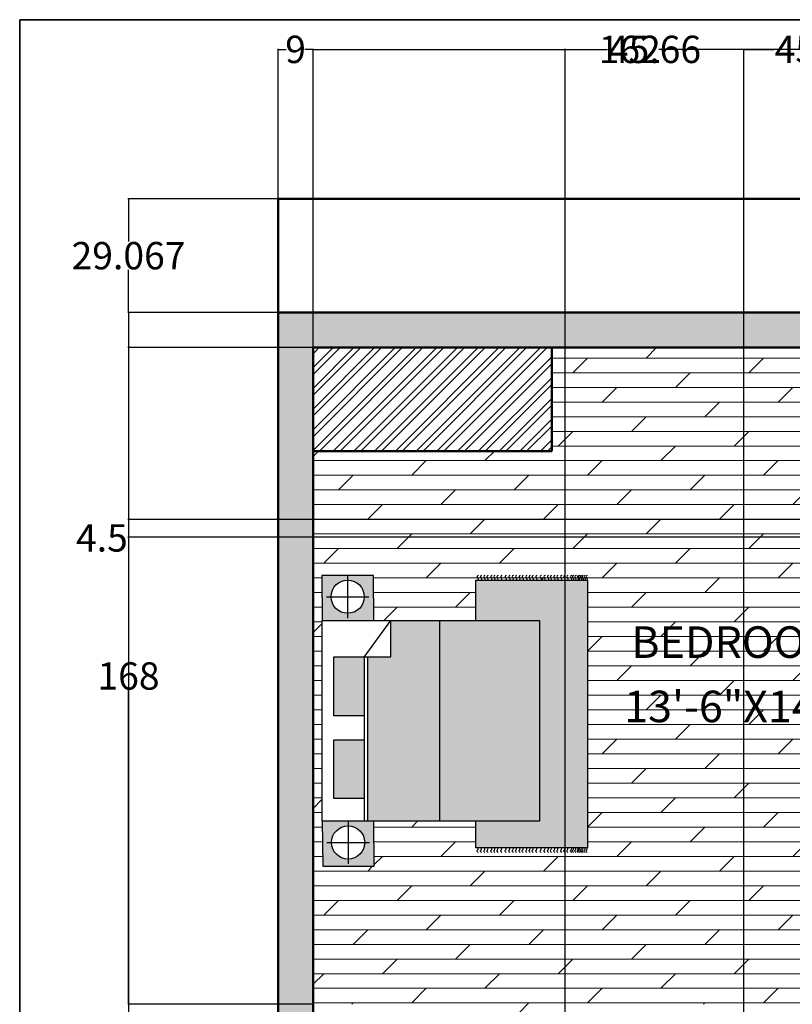
# Model space of a CAD drawing. Units: inches. Extents: x 1381 to 2246, y 1317 to 2168.
# Tile 6 of 15: x 1381 to 1579, y 1916 to 2168. Entities that reach past the tile are written whole.
import ezdxf

# ---------------------------------------------------------------- set-up
doc = ezdxf.new("R2010")
doc.units = ezdxf.units.IN
doc.header["$MEASUREMENT"] = 0
for name, color, linetype, lineweight in [('A-ANNO-DIMS', 2, 'Continuous', 18), ('A-ANNO-TTLB', 7, 'Continuous', 35), ('A-AREA-IDEN', 3, 'Continuous', 25), ('A-FLOR-PATT', 252, 'Continuous', 13), ('A-FURN', 8, 'Continuous', 18), ('A-GLAZ', 4, 'Continuous', 25), ('A-WALL', 7, 'Continuous', 50)]:
    doc.layers.add(name, color=color, linetype=linetype, lineweight=lineweight)
doc.layers.add('furniture', color=250, linetype='Continuous')
doc.styles.get("Standard").update_dxf_attribs({"font": 'arial.ttf'})
doc.dimstyles.get("Standard").update_dxf_attribs({"dimtxt": 7, "dimasz": 0.18, "dimexe": 0.18, "dimexo": 0.0625, "dimgap": 0.09, "dimtad": 0, "dimtih": 1, "dimtoh": 1, "dimdec": 1, "dimzin": 0, "dimdsep": 46, "dimlunit": 3, "dimtxsty": 'Standard', "dimcen": 0.09, "dimadec": 0, "dimazin": 0, "dimtfac": 1, "dimtdec": 1, "dimtofl": 0, "dimtmove": 0, "dimatfit": 3, "dimfxl": 1, "dimtolj": 1, "dimtzin": 0, "dimarcsym": 0})

# ---------------------------------------------------------------- blocks, each defined once
blk = doc.blocks.new('CARPET')
at = {"layer": 'furniture'}
for p, q in [((-51.53, -98.11), (-51.53, -55.12)), ((-51.53, -55.12), (-41.27, -55.12)), ((36, -55.12), (51.55, -55.12)), ((51.55, -55.12), (51.55, -98.11)), ((51.55, -98.11), (-51.53, -98.11))]:
    blk.add_line(p, q, dxfattribs=at)
for points, knots in [([(-53.37, -55.99), (-53.22, -55.8), (-52.9, -55.41), (-52.34, -55.8), (-51.89, -56.08), (-51.65, -55.91), (-51.53, -55.83)], [0, 0, 0, 0, 0.653278, 1.290138, 1.740457, 2.114451, 2.114451, 2.114451, 2.114451]), ([(-53.37, -57.26), (-53.22, -57.07), (-52.9, -56.67), (-52.34, -57.07), (-51.89, -57.35), (-51.65, -57.17), (-51.53, -57.1)], [0, 0, 0, 0, 0.653278, 1.290138, 1.740457, 2.114451, 2.114451, 2.114451, 2.114451]), ([(53.37, -55.99), (53.22, -55.8), (52.9, -55.41), (52.34, -55.8), (51.89, -56.08), (51.65, -55.91), (51.53, -55.83)], [0, 0, 0, 0, 0.653278, 1.290138, 1.740457, 2.114451, 2.114451, 2.114451, 2.114451]), ([(53.37, -57.26), (53.22, -57.07), (52.9, -56.67), (52.34, -57.07), (51.89, -57.35), (51.65, -57.17), (51.53, -57.1)], [0, 0, 0, 0, 0.653278, 1.290138, 1.740457, 2.114451, 2.114451, 2.114451, 2.114451]), ([(-53.37, -58.59), (-53.22, -58.4), (-52.9, -58.01), (-52.34, -58.4), (-51.89, -58.68), (-51.65, -58.5), (-51.53, -58.43)], [0, 0, 0, 0, 0.653278, 1.290138, 1.740457, 2.114451, 2.114451, 2.114451, 2.114451]), ([(-53.37, -59.78), (-53.22, -59.58), (-52.9, -59.19), (-52.34, -59.58), (-51.89, -59.86), (-51.65, -59.69), (-51.53, -59.61)], [0, 0, 0, 0, 0.653278, 1.290138, 1.740457, 2.114451, 2.114451, 2.114451, 2.114451]), ([(53.37, -58.59), (53.22, -58.4), (52.9, -58.01), (52.34, -58.4), (51.89, -58.68), (51.65, -58.5), (51.53, -58.43)], [0, 0, 0, 0, 0.653278, 1.290138, 1.740457, 2.114451, 2.114451, 2.114451, 2.114451]), ([(53.37, -59.78), (53.22, -59.58), (52.9, -59.19), (52.34, -59.58), (51.89, -59.86), (51.65, -59.69), (51.53, -59.61)], [0, 0, 0, 0, 0.653278, 1.290138, 1.740457, 2.114451, 2.114451, 2.114451, 2.114451]), ([(-53.37, -61.22), (-53.22, -61.02), (-52.9, -60.63), (-52.34, -61.02), (-51.89, -61.3), (-51.65, -61.13), (-51.53, -61.05)], [0, 0, 0, 0, 0.653278, 1.290138, 1.740457, 2.114451, 2.114451, 2.114451, 2.114451]), ([(-53.37, -62.44), (-53.22, -62.25), (-52.9, -61.86), (-52.34, -62.25), (-51.89, -62.53), (-51.65, -62.36), (-51.53, -62.28)], [0, 0, 0, 0, 0.653278, 1.290138, 1.740457, 2.114451, 2.114451, 2.114451, 2.114451]), ([(-53.37, -63.63), (-53.22, -63.43), (-52.9, -63.04), (-52.34, -63.43), (-51.89, -63.72), (-51.65, -63.54), (-51.53, -63.46)], [0, 0, 0, 0, 0.653278, 1.290138, 1.740457, 2.114451, 2.114451, 2.114451, 2.114451]), ([(53.37, -61.22), (53.22, -61.02), (52.9, -60.63), (52.34, -61.02), (51.89, -61.3), (51.65, -61.13), (51.53, -61.05)], [0, 0, 0, 0, 0.653278, 1.290138, 1.740457, 2.114451, 2.114451, 2.114451, 2.114451]), ([(53.37, -62.44), (53.22, -62.25), (52.9, -61.86), (52.34, -62.25), (51.89, -62.53), (51.65, -62.36), (51.53, -62.28)], [0, 0, 0, 0, 0.653278, 1.290138, 1.740457, 2.114451, 2.114451, 2.114451, 2.114451]), ([(53.37, -63.63), (53.22, -63.43), (52.9, -63.04), (52.34, -63.43), (51.89, -63.72), (51.65, -63.54), (51.53, -63.46)], [0, 0, 0, 0, 0.653278, 1.290138, 1.740457, 2.114451, 2.114451, 2.114451, 2.114451]), ([(-53.37, -65.07), (-53.22, -64.87), (-52.9, -64.48), (-52.34, -64.87), (-51.89, -65.15), (-51.65, -64.98), (-51.53, -64.9)], [0, 0, 0, 0, 0.653278, 1.290138, 1.740457, 2.114451, 2.114451, 2.114451, 2.114451]), ([(-53.37, -66.76), (-53.22, -66.56), (-52.9, -66.17), (-52.34, -66.56), (-51.89, -66.84), (-51.65, -66.67), (-51.53, -66.59)], [0, 0, 0, 0, 0.653278, 1.290138, 1.740457, 2.114451, 2.114451, 2.114451, 2.114451]), ([(-53.37, -68.2), (-53.22, -68), (-52.9, -67.61), (-52.34, -68), (-51.89, -68.28), (-51.65, -68.11), (-51.53, -68.03)], [0, 0, 0, 0, 0.653278, 1.290138, 1.740457, 2.114451, 2.114451, 2.114451, 2.114451]), ([(53.37, -65.07), (53.22, -64.87), (52.9, -64.48), (52.34, -64.87), (51.89, -65.15), (51.65, -64.98), (51.53, -64.9)], [0, 0, 0, 0, 0.653278, 1.290138, 1.740457, 2.114451, 2.114451, 2.114451, 2.114451]), ([(53.37, -66.76), (53.22, -66.56), (52.9, -66.17), (52.34, -66.56), (51.89, -66.84), (51.65, -66.67), (51.53, -66.59)], [0, 0, 0, 0, 0.653278, 1.290138, 1.740457, 2.114451, 2.114451, 2.114451, 2.114451]), ([(53.37, -68.2), (53.22, -68), (52.9, -67.61), (52.34, -68), (51.89, -68.28), (51.65, -68.11), (51.53, -68.03)], [0, 0, 0, 0, 0.653278, 1.290138, 1.740457, 2.114451, 2.114451, 2.114451, 2.114451]), ([(-53.37, -69.53), (-53.22, -69.33), (-52.9, -68.94), (-52.34, -69.33), (-51.89, -69.61), (-51.65, -69.44), (-51.53, -69.36)], [0, 0, 0, 0, 0.653278, 1.290138, 1.740457, 2.114451, 2.114451, 2.114451, 2.114451]), ([(-53.37, -70.79), (-53.22, -70.6), (-52.9, -70.21), (-52.34, -70.6), (-51.89, -70.88), (-51.65, -70.7), (-51.53, -70.63)], [0, 0, 0, 0, 0.653278, 1.290138, 1.740457, 2.114451, 2.114451, 2.114451, 2.114451]), ([(-53.37, -72.12), (-53.22, -71.93), (-52.9, -71.54), (-52.34, -71.93), (-51.89, -72.21), (-51.65, -72.04), (-51.53, -71.96)], [0, 0, 0, 0, 0.653278, 1.290138, 1.740457, 2.114451, 2.114451, 2.114451, 2.114451]), ([(53.37, -69.53), (53.22, -69.33), (52.9, -68.94), (52.34, -69.33), (51.89, -69.61), (51.65, -69.44), (51.53, -69.36)], [0, 0, 0, 0, 0.653278, 1.290138, 1.740457, 2.114451, 2.114451, 2.114451, 2.114451]), ([(53.37, -70.79), (53.22, -70.6), (52.9, -70.21), (52.34, -70.6), (51.89, -70.88), (51.65, -70.7), (51.53, -70.63)], [0, 0, 0, 0, 0.653278, 1.290138, 1.740457, 2.114451, 2.114451, 2.114451, 2.114451]), ([(53.37, -72.12), (53.22, -71.93), (52.9, -71.54), (52.34, -71.93), (51.89, -72.21), (51.65, -72.04), (51.53, -71.96)], [0, 0, 0, 0, 0.653278, 1.290138, 1.740457, 2.114451, 2.114451, 2.114451, 2.114451]), ([(-53.37, -73.31), (-53.22, -73.11), (-52.9, -72.72), (-52.34, -73.11), (-51.89, -73.4), (-51.65, -73.22), (-51.53, -73.14)], [0, 0, 0, 0, 0.653278, 1.290138, 1.740457, 2.114451, 2.114451, 2.114451, 2.114451]), ([(-53.37, -74.75), (-53.22, -74.55), (-52.9, -74.16), (-52.34, -74.55), (-51.89, -74.83), (-51.65, -74.66), (-51.53, -74.58)], [0, 0, 0, 0, 0.653278, 1.290138, 1.740457, 2.114451, 2.114451, 2.114451, 2.114451]), ([(-53.37, -75.98), (-53.22, -75.78), (-52.9, -75.39), (-52.34, -75.78), (-51.89, -76.06), (-51.65, -75.89), (-51.53, -75.81)], [0, 0, 0, 0, 0.653278, 1.290138, 1.740457, 2.114451, 2.114451, 2.114451, 2.114451]), ([(53.37, -73.31), (53.22, -73.11), (52.9, -72.72), (52.34, -73.11), (51.89, -73.4), (51.65, -73.22), (51.53, -73.14)], [0, 0, 0, 0, 0.653278, 1.290138, 1.740457, 2.114451, 2.114451, 2.114451, 2.114451]), ([(53.37, -74.75), (53.22, -74.55), (52.9, -74.16), (52.34, -74.55), (51.89, -74.83), (51.65, -74.66), (51.53, -74.58)], [0, 0, 0, 0, 0.653278, 1.290138, 1.740457, 2.114451, 2.114451, 2.114451, 2.114451]), ([(53.37, -75.98), (53.22, -75.78), (52.9, -75.39), (52.34, -75.78), (51.89, -76.06), (51.65, -75.89), (51.53, -75.81)], [0, 0, 0, 0, 0.653278, 1.290138, 1.740457, 2.114451, 2.114451, 2.114451, 2.114451]), ([(-53.37, -77.16), (-53.22, -76.96), (-52.9, -76.57), (-52.34, -76.96), (-51.89, -77.25), (-51.65, -77.07), (-51.53, -76.99)], [0, 0, 0, 0, 0.653278, 1.290138, 1.740457, 2.114451, 2.114451, 2.114451, 2.114451]), ([(-53.37, -78.6), (-53.22, -78.4), (-52.9, -78.01), (-52.34, -78.4), (-51.89, -78.68), (-51.65, -78.51), (-51.53, -78.43)], [0, 0, 0, 0, 0.653278, 1.290138, 1.740457, 2.114451, 2.114451, 2.114451, 2.114451]), ([(53.37, -77.16), (53.22, -76.96), (52.9, -76.57), (52.34, -76.96), (51.89, -77.25), (51.65, -77.07), (51.53, -76.99)], [0, 0, 0, 0, 0.653278, 1.290138, 1.740457, 2.114451, 2.114451, 2.114451, 2.114451]), ([(53.37, -78.6), (53.22, -78.4), (52.9, -78.01), (52.34, -78.4), (51.89, -78.68), (51.65, -78.51), (51.53, -78.43)], [0, 0, 0, 0, 0.653278, 1.290138, 1.740457, 2.114451, 2.114451, 2.114451, 2.114451]), ([(-53.37, -80.29), (-53.22, -80.09), (-52.9, -79.7), (-52.34, -80.09), (-51.89, -80.37), (-51.65, -80.2), (-51.53, -80.12)], [0, 0, 0, 0, 0.653278, 1.290138, 1.740457, 2.114451, 2.114451, 2.114451, 2.114451]), ([(-53.37, -81.73), (-53.22, -81.53), (-52.9, -81.14), (-52.34, -81.53), (-51.89, -81.81), (-51.65, -81.64), (-51.53, -81.56)], [0, 0, 0, 0, 0.653278, 1.290138, 1.740457, 2.114451, 2.114451, 2.114451, 2.114451]), ([(-53.37, -83.06), (-53.22, -82.86), (-52.9, -82.47), (-52.34, -82.86), (-51.89, -83.14), (-51.65, -82.97), (-51.53, -82.89)], [0, 0, 0, 0, 0.653278, 1.290138, 1.740457, 2.114451, 2.114451, 2.114451, 2.114451]), ([(53.37, -80.29), (53.22, -80.09), (52.9, -79.7), (52.34, -80.09), (51.89, -80.37), (51.65, -80.2), (51.53, -80.12)], [0, 0, 0, 0, 0.653278, 1.290138, 1.740457, 2.114451, 2.114451, 2.114451, 2.114451]), ([(53.37, -81.73), (53.22, -81.53), (52.9, -81.14), (52.34, -81.53), (51.89, -81.81), (51.65, -81.64), (51.53, -81.56)], [0, 0, 0, 0, 0.653278, 1.290138, 1.740457, 2.114451, 2.114451, 2.114451, 2.114451]), ([(53.37, -83.06), (53.22, -82.86), (52.9, -82.47), (52.34, -82.86), (51.89, -83.14), (51.65, -82.97), (51.53, -82.89)], [0, 0, 0, 0, 0.653278, 1.290138, 1.740457, 2.114451, 2.114451, 2.114451, 2.114451]), ([(-53.37, -84.18), (-53.22, -83.99), (-52.9, -83.6), (-52.34, -83.99), (-51.89, -84.27), (-51.65, -84.09), (-51.53, -84.02)], [0, 0, 0, 0, 0.653278, 1.290138, 1.740457, 2.114451, 2.114451, 2.114451, 2.114451]), ([(-53.37, -85.51), (-53.22, -85.32), (-52.9, -84.93), (-52.34, -85.32), (-51.89, -85.6), (-51.65, -85.42), (-51.53, -85.35)], [0, 0, 0, 0, 0.653278, 1.290138, 1.740457, 2.114451, 2.114451, 2.114451, 2.114451]), ([(-53.37, -86.7), (-53.22, -86.5), (-52.9, -86.11), (-52.34, -86.5), (-51.89, -86.78), (-51.65, -86.61), (-51.53, -86.53)], [0, 0, 0, 0, 0.653278, 1.290138, 1.740457, 2.114451, 2.114451, 2.114451, 2.114451]), ([(53.37, -84.18), (53.22, -83.99), (52.9, -83.6), (52.34, -83.99), (51.89, -84.27), (51.65, -84.09), (51.53, -84.02)], [0, 0, 0, 0, 0.653278, 1.290138, 1.740457, 2.114451, 2.114451, 2.114451, 2.114451]), ([(53.37, -85.51), (53.22, -85.32), (52.9, -84.93), (52.34, -85.32), (51.89, -85.6), (51.65, -85.42), (51.53, -85.35)], [0, 0, 0, 0, 0.653278, 1.290138, 1.740457, 2.114451, 2.114451, 2.114451, 2.114451]), ([(53.37, -86.7), (53.22, -86.5), (52.9, -86.11), (52.34, -86.5), (51.89, -86.78), (51.65, -86.61), (51.53, -86.53)], [0, 0, 0, 0, 0.653278, 1.290138, 1.740457, 2.114451, 2.114451, 2.114451, 2.114451]), ([(-53.37, -88.14), (-53.22, -87.94), (-52.9, -87.55), (-52.34, -87.94), (-51.89, -88.22), (-51.65, -88.05), (-51.53, -87.97)], [0, 0, 0, 0, 0.653278, 1.290138, 1.740457, 2.114451, 2.114451, 2.114451, 2.114451]), ([(-53.37, -89.36), (-53.22, -89.17), (-52.9, -88.78), (-52.34, -89.17), (-51.89, -89.45), (-51.65, -89.28), (-51.53, -89.2)], [0, 0, 0, 0, 0.653278, 1.290138, 1.740457, 2.114451, 2.114451, 2.114451, 2.114451]), ([(-53.37, -90.55), (-53.22, -90.35), (-52.9, -89.96), (-52.34, -90.35), (-51.89, -90.64), (-51.65, -90.46), (-51.53, -90.38)], [0, 0, 0, 0, 0.653278, 1.290138, 1.740457, 2.114451, 2.114451, 2.114451, 2.114451]), ([(53.37, -88.14), (53.22, -87.94), (52.9, -87.55), (52.34, -87.94), (51.89, -88.22), (51.65, -88.05), (51.53, -87.97)], [0, 0, 0, 0, 0.653278, 1.290138, 1.740457, 2.114451, 2.114451, 2.114451, 2.114451]), ([(53.37, -89.36), (53.22, -89.17), (52.9, -88.78), (52.34, -89.17), (51.89, -89.45), (51.65, -89.28), (51.53, -89.2)], [0, 0, 0, 0, 0.653278, 1.290138, 1.740457, 2.114451, 2.114451, 2.114451, 2.114451]), ([(53.37, -90.55), (53.22, -90.35), (52.9, -89.96), (52.34, -90.35), (51.9, -90.63), (51.66, -90.47), (51.55, -90.4)], [0, 0, 0, 0, 0.653278, 1.290138, 1.740457, 2.0926, 2.0926, 2.0926, 2.0926]), ([(-53.37, -91.99), (-53.22, -91.79), (-52.9, -91.4), (-52.34, -91.79), (-51.89, -92.07), (-51.65, -91.9), (-51.53, -91.82)], [0, 0, 0, 0, 0.653278, 1.290138, 1.740457, 2.114451, 2.114451, 2.114451, 2.114451]), ([(-53.37, -92.69), (-53.22, -92.48), (-52.9, -92.08), (-52.35, -92.49), (-51.89, -92.77), (-51.65, -92.6), (-51.53, -92.52)], [0, 0, 0, 0, 0.663904, 1.307406, 1.757725, 2.131719, 2.131719, 2.131719, 2.131719]), ([(-53.37, -93.61), (-53.22, -93.42), (-52.9, -93.03), (-52.34, -93.42), (-51.89, -93.7), (-51.65, -93.52), (-51.53, -93.45)], [0, 0, 0, 0, 0.653278, 1.290138, 1.740457, 2.114451, 2.114451, 2.114451, 2.114451]), ([(-53.37, -94.55), (-53.22, -94.35), (-52.9, -93.96), (-52.34, -94.35), (-51.89, -94.63), (-51.65, -94.46), (-51.53, -94.38)], [0, 0, 0, 0, 0.653278, 1.290138, 1.740457, 2.114451, 2.114451, 2.114451, 2.114451]), ([(-53.37, -95.05), (-53.22, -94.85), (-52.9, -94.46), (-52.34, -94.85), (-51.89, -95.14), (-51.65, -94.96), (-51.53, -94.88)], [0, 0, 0, 0, 0.653278, 1.290138, 1.740457, 2.114451, 2.114451, 2.114451, 2.114451]), ([(53.37, -91.99), (53.22, -91.79), (52.9, -91.4), (52.34, -91.79), (51.9, -92.07), (51.66, -91.91), (51.55, -91.83)], [0, 0, 0, 0, 0.653278, 1.290138, 1.740457, 2.0926, 2.0926, 2.0926, 2.0926]), ([(53.37, -92.69), (53.22, -92.49), (52.9, -92.09), (52.34, -92.49), (51.9, -92.77), (51.66, -92.61), (51.55, -92.53)], [0, 0, 0, 0, 0.656792, 1.295826, 1.746145, 2.098292, 2.098292, 2.098292, 2.098292]), ([(53.37, -93.66), (53.22, -93.46), (52.9, -93.07), (52.34, -93.46), (51.9, -93.74), (51.66, -93.58), (51.55, -93.5)], [0, 0, 0, 0, 0.653278, 1.290138, 1.740457, 2.0926, 2.0926, 2.0926, 2.0926]), ([(53.37, -94.59), (53.22, -94.4), (52.9, -94.01), (52.34, -94.4), (51.9, -94.68), (51.66, -94.51), (51.55, -94.44)], [0, 0, 0, 0, 0.653278, 1.290138, 1.740457, 2.0926, 2.0926, 2.0926, 2.0926]), ([(53.37, -95.1), (53.22, -94.9), (52.9, -94.51), (52.34, -94.9), (51.9, -95.18), (51.66, -95.02), (51.55, -94.94)], [0, 0, 0, 0, 0.653278, 1.290138, 1.740457, 2.0926, 2.0926, 2.0926, 2.0926]), ([(-53.37, -95.73), (-53.22, -95.54), (-52.9, -95.15), (-52.34, -95.54), (-51.89, -95.82), (-51.65, -95.65), (-51.53, -95.57)], [0, 0, 0, 0, 0.653278, 1.290138, 1.740457, 2.114451, 2.114451, 2.114451, 2.114451]), ([(-53.37, -96.38), (-53.22, -96.18), (-52.9, -95.79), (-52.34, -96.18), (-51.89, -96.47), (-51.65, -96.29), (-51.53, -96.21)], [0, 0, 0, 0, 0.653278, 1.290138, 1.740457, 2.114451, 2.114451, 2.114451, 2.114451]), ([(-53.37, -97.17), (-53.22, -96.98), (-52.9, -96.59), (-52.34, -96.98), (-51.89, -97.26), (-51.65, -97.08), (-51.53, -97.01)], [0, 0, 0, 0, 0.653278, 1.290138, 1.740457, 2.114451, 2.114451, 2.114451, 2.114451]), ([(-53.37, -97.99), (-53.22, -97.79), (-52.9, -97.4), (-52.34, -97.79), (-51.89, -98.08), (-51.65, -97.9), (-51.53, -97.82)], [0, 0, 0, 0, 0.653278, 1.290138, 1.740457, 2.114451, 2.114451, 2.114451, 2.114451]), ([(53.37, -95.78), (53.22, -95.58), (52.9, -95.19), (52.34, -95.58), (51.89, -95.86), (51.65, -95.69), (51.53, -95.61)], [0, 0, 0, 0, 0.653278, 1.290138, 1.740457, 2.114451, 2.114451, 2.114451, 2.114451]), ([(53.37, -96.43), (53.22, -96.23), (52.9, -95.84), (52.34, -96.23), (51.89, -96.51), (51.65, -96.34), (51.53, -96.26)], [0, 0, 0, 0, 0.653278, 1.290138, 1.740457, 2.114451, 2.114451, 2.114451, 2.114451]), ([(53.37, -97.22), (53.22, -97.02), (52.9, -96.63), (52.34, -97.02), (51.89, -97.3), (51.65, -97.13), (51.53, -97.05)], [0, 0, 0, 0, 0.653278, 1.290138, 1.740457, 2.114451, 2.114451, 2.114451, 2.114451]), ([(53.37, -97.99), (53.22, -97.79), (52.9, -97.4), (52.34, -97.79), (51.89, -98.08), (51.65, -97.9), (51.53, -97.82)], [0, 0, 0, 0, 0.653278, 1.290138, 1.740457, 2.114451, 2.114451, 2.114451, 2.114451])]:
    blk.add_open_spline(points, degree=3, knots=knots, dxfattribs=at)
blk = doc.blocks.new('A$C58D270C6')
at = {"layer": 'furniture'}
for p, q in [((9.09, 124.13), (9.09, 108.87)), ((1.46, 116.5), (16.73, 116.5)), ((14.97, 94.84), (24.62, 107.92)), ((24.62, 94.93), (24.62, 107.92)), ((42.08, 108), (42.08, 36)), ((14.97, 94.93), (24.62, 94.93)), ((14.97, 94.84), (14.97, 36)), ((16.22, 94.93), (16.22, 36)), ((9.25, 36), (9.25, 20.74)), ((1.62, 28.37), (16.88, 28.37))]:
    blk.add_line(p, q, dxfattribs=at)
for points in [[(18.5, 108), (18.34, 124.13), (-0.16, 124.13), (0, 108)], [(0, 108), (77.91, 108), (77.91, 36), (0, 36)], [(4.09, 94.93), (14.97, 94.93), (14.97, 73.83), (4.09, 73.83)], [(4.09, 65.23), (14.97, 65.23), (14.97, 44.13), (4.09, 44.13)], [(18.65, 19.87), (18.5, 36), (0, 36), (0.16, 19.87)]]:
    blk.add_lwpolyline(points, close=True, dxfattribs=at)
for centre in [(9.09, 116.5), (9.25, 28.37)]:
    blk.add_circle(centre, 5.95, dxfattribs=at)
at = {"layer": 'furniture', "xscale": 0.9312884925094044, "yscale": 0.9312884925094044, "zscale": 0.9312884925094044, "rotation": 90}
blk.add_blockref('CARPET', (3.79, 74.47), dxfattribs=at)
blk = doc.blocks.new('*D50')
at = {"layer": 'A-ANNO-DIMS', "color": 0, "lineweight": -2, "transparency": 16777216}
for p, q in [((1446.99, 2092.92), (1408.62, 2092.92)), ((1408.8, 2092.74), (1408.8, 1786.08)), ((1408.8, 1472.1), (1408.8, 1778.75)), ((1446.99, 1471.92), (1408.62, 1471.92))]:
    blk.add_line(p, q, dxfattribs=at)
at = {"layer": 'A-ANNO-DIMS', "color": 0, "transparency": 16777216}
for points in [[(1408.77, 2092.74), (1408.83, 2092.74), (1408.8, 2092.92)], [(1408.77, 1472.1), (1408.83, 1472.1), (1408.8, 1471.92)]]:
    blk.add_solid(points, dxfattribs=at)
at = {"layer": 'Defpoints', "color": 0, "transparency": 16777216}
for p in [(1408.8, 2092.92), (1447.05, 2092.92), (1447.05, 1471.92)]:
    blk.add_point(p, dxfattribs=at)
at = {"layer": 'A-ANNO-DIMS', "color": 0, "transparency": 16777216, "insert": (1408.8, 1782.42), "char_height": 7, "attachment_point": 5}
blk.add_mtext('\\A1;621', dxfattribs=at)
blk = doc.blocks.new('*D51')
at = {"layer": 'A-ANNO-DIMS', "color": 0, "lineweight": -2, "transparency": 16777216}
for p, q in [((1446.99, 2121.98), (1408.62, 2121.98)), ((1408.8, 2121.8), (1408.8, 2111.11)), ((1408.8, 2093.1), (1408.8, 2103.79)), ((1446.99, 2092.92), (1408.62, 2092.92))]:
    blk.add_line(p, q, dxfattribs=at)
at = {"layer": 'A-ANNO-DIMS', "color": 0, "transparency": 16777216}
for points in [[(1408.77, 2121.8), (1408.83, 2121.8), (1408.8, 2121.98)], [(1408.77, 2093.1), (1408.83, 2093.1), (1408.8, 2092.92)]]:
    blk.add_solid(points, dxfattribs=at)
at = {"layer": 'Defpoints', "color": 0, "transparency": 16777216}
for p in [(1408.8, 2121.98), (1447.05, 2121.98), (1447.05, 2092.92)]:
    blk.add_point(p, dxfattribs=at)
at = {"layer": 'A-ANNO-DIMS', "color": 0, "transparency": 16777216, "insert": (1408.8, 2107.45), "char_height": 7, "attachment_point": 5}
blk.add_mtext('\\A1;29.067', dxfattribs=at)
blk = doc.blocks.new('*D53')
at = {"layer": 'A-ANNO-DIMS', "color": 0, "lineweight": -2, "transparency": 16777216}
for p, q in [((1447.05, 2092.98), (1447.05, 2160.41)), ((1447.23, 2160.23), (1449.16, 2160.23)), ((1455.87, 2160.23), (1453.94, 2160.23)), ((1456.05, 2083.98), (1456.05, 2160.41))]:
    blk.add_line(p, q, dxfattribs=at)
at = {"layer": 'A-ANNO-DIMS', "color": 0, "transparency": 16777216}
for points in [[(1447.23, 2160.26), (1447.23, 2160.2), (1447.05, 2160.23)], [(1455.87, 2160.26), (1455.87, 2160.2), (1456.05, 2160.23)]]:
    blk.add_solid(points, dxfattribs=at)
at = {"layer": 'Defpoints', "color": 0, "transparency": 16777216}
for p in [(1456.05, 2160.23), (1447.05, 2092.92), (1456.05, 2083.92)]:
    blk.add_point(p, dxfattribs=at)
at = {"layer": 'A-ANNO-DIMS', "color": 0, "transparency": 16777216, "insert": (1451.55, 2160.23), "char_height": 7, "attachment_point": 5}
blk.add_mtext('\\A1;9', dxfattribs=at)
blk = doc.blocks.new('*D57')
at = {"layer": 'A-ANNO-DIMS', "color": 0, "lineweight": -2, "transparency": 16777216}
for p, q in [((1455.99, 2083.92), (1408.62, 2083.92)), ((1408.8, 2083.74), (1408.8, 2003.58)), ((1408.8, 1916.1), (1408.8, 1996.25)), ((1455.99, 1915.92), (1408.62, 1915.92))]:
    blk.add_line(p, q, dxfattribs=at)
at = {"layer": 'A-ANNO-DIMS', "color": 0, "transparency": 16777216}
for points in [[(1408.77, 2083.74), (1408.83, 2083.74), (1408.8, 2083.92)], [(1408.77, 1916.1), (1408.83, 1916.1), (1408.8, 1915.92)]]:
    blk.add_solid(points, dxfattribs=at)
at = {"layer": 'Defpoints', "color": 0, "transparency": 16777216}
for p in [(1408.8, 2083.92), (1456.05, 2083.92), (1456.05, 1915.92)]:
    blk.add_point(p, dxfattribs=at)
at = {"layer": 'A-ANNO-DIMS', "color": 0, "transparency": 16777216, "insert": (1408.8, 1999.92), "char_height": 7, "attachment_point": 5}
blk.add_mtext('\\A1;168', dxfattribs=at)
blk = doc.blocks.new('*D58')
at = {"layer": 'A-ANNO-DIMS', "color": 0, "lineweight": -2, "transparency": 16777216}
for p, q in [((1456.05, 2083.98), (1456.05, 2160.41)), ((1456.23, 2160.23), (1529.59, 2160.23)), ((1617.87, 2160.23), (1544.51, 2160.23)), ((1618.05, 2083.98), (1618.05, 2160.41))]:
    blk.add_line(p, q, dxfattribs=at)
at = {"layer": 'A-ANNO-DIMS', "color": 0, "transparency": 16777216}
for points in [[(1456.23, 2160.26), (1456.23, 2160.2), (1456.05, 2160.23)], [(1617.87, 2160.26), (1617.87, 2160.2), (1618.05, 2160.23)]]:
    blk.add_solid(points, dxfattribs=at)
at = {"layer": 'Defpoints', "color": 0, "transparency": 16777216}
for p in [(1618.05, 2160.23), (1456.05, 2083.92), (1618.05, 2083.92)]:
    blk.add_point(p, dxfattribs=at)
at = {"layer": 'A-ANNO-DIMS', "color": 0, "transparency": 16777216, "insert": (1537.05, 2160.23), "char_height": 7, "attachment_point": 5}
blk.add_mtext('\\A1;162', dxfattribs=at)
blk = doc.blocks.new('*D70')
at = {"layer": 'A-ANNO-DIMS', "color": 0, "lineweight": -2, "transparency": 16777216}
for p, q in [((1655.76, 2039.92), (1408.62, 2039.92)), ((1408.8, 2039.74), (1408.8, 2035.6)), ((1655.76, 2035.42), (1408.62, 2035.42)), ((1408.8, 2035.42), (1408.8, 2035.24)), ((1408.8, 2035.24), (1408.62, 2035.24))]:
    blk.add_line(p, q, dxfattribs=at)
at = {"layer": 'A-ANNO-DIMS', "color": 0, "transparency": 16777216}
for points in [[(1408.77, 2039.74), (1408.83, 2039.74), (1408.8, 2039.92)], [(1408.77, 2035.6), (1408.83, 2035.6), (1408.8, 2035.42)]]:
    blk.add_solid(points, dxfattribs=at)
at = {"layer": 'Defpoints', "color": 0, "transparency": 16777216}
for p in [(1655.82, 2039.92), (1408.8, 2035.42), (1655.82, 2035.42)]:
    blk.add_point(p, dxfattribs=at)
at = {"layer": 'A-ANNO-DIMS', "color": 0, "transparency": 16777216, "insert": (1401.99, 2035.24), "char_height": 7, "attachment_point": 5}
blk.add_mtext('\\A1;4.5', dxfattribs=at)
blk = doc.blocks.new('*D71')
at = {"layer": 'A-ANNO-DIMS', "color": 0, "lineweight": -2, "transparency": 16777216}
for p, q in [((1520.55, 1911.48), (1520.55, 2160.41)), ((1520.73, 2160.23), (1531.34, 2160.23)), ((1566.03, 2160.23), (1555.42, 2160.23)), ((1566.21, 1911.48), (1566.21, 2160.41))]:
    blk.add_line(p, q, dxfattribs=at)
at = {"layer": 'A-ANNO-DIMS', "color": 0, "transparency": 16777216}
for points in [[(1520.73, 2160.26), (1520.73, 2160.2), (1520.55, 2160.23)], [(1566.03, 2160.26), (1566.03, 2160.2), (1566.21, 2160.23)]]:
    blk.add_solid(points, dxfattribs=at)
at = {"layer": 'Defpoints', "color": 0, "transparency": 16777216}
for p in [(1566.21, 2160.23), (1520.55, 1911.42), (1566.21, 1911.42)]:
    blk.add_point(p, dxfattribs=at)
at = {"layer": 'A-ANNO-DIMS', "color": 0, "transparency": 16777216, "insert": (1543.38, 2160.23), "char_height": 7, "attachment_point": 5}
blk.add_mtext('\\A1;45.66', dxfattribs=at)
blk = doc.blocks.new('*D72')
at = {"layer": 'A-ANNO-DIMS', "color": 0, "lineweight": -2, "transparency": 16777216}
for p, q in [((1566.21, 1911.48), (1566.21, 2160.41)), ((1566.39, 2160.23), (1573.94, 2160.23)), ((1611.06, 2160.23), (1603.51, 2160.23)), ((1611.24, 1911.48), (1611.24, 2160.41))]:
    blk.add_line(p, q, dxfattribs=at)
at = {"layer": 'A-ANNO-DIMS', "color": 0, "transparency": 16777216}
for points in [[(1566.39, 2160.26), (1566.39, 2160.2), (1566.21, 2160.23)], [(1611.06, 2160.26), (1611.06, 2160.2), (1611.24, 2160.23)]]:
    blk.add_solid(points, dxfattribs=at)
at = {"layer": 'Defpoints', "color": 0, "transparency": 16777216}
for p in [(1611.24, 2160.23), (1566.21, 1911.42), (1611.24, 1911.42)]:
    blk.add_point(p, dxfattribs=at)
at = {"layer": 'A-ANNO-DIMS', "color": 0, "transparency": 16777216, "insert": (1588.72, 2160.23), "char_height": 7, "attachment_point": 5}
blk.add_mtext('\\A1;45.025', dxfattribs=at)

msp = doc.modelspace()

# ---------------------------------------------------------------- hatches: boundary and pattern name
at = {"layer": 'A-FLOR-PATT'}
h = msp.add_hatch(dxfattribs=at)
h.set_pattern_fill('ANSI32', color=256, scale=10)
h.set_pattern_definition([(45, (-5e-13, 373.5), (-2.6516504, 2.6516504), []), (45, (1.7678, 373.5), (-2.6516504, 2.6516504), [])])
h.paths.add_polyline_path([(1517.1194, 2083.9163), (1456.051, 2083.9163), (1456.051, 2057.4148), (1517.1194, 2057.4148)])
h = msp.add_hatch(dxfattribs=at)
h.set_pattern_fill('DOLMIT', color=256, scale=15)
h.paths.add_polyline_path([(1618.051, 2040.2358), (1618.051, 2083.9163), (1517.1194, 2083.9163), (1517.1194, 2057.4148), (1456.051, 2057.4148), (1456.051, 1915.9163), (1478.9621, 1915.9163), (1478.9621, 1913.6663), (1511.016, 1913.6663), (1511.016, 1915.9163), (1566.2107, 1915.9163), (1566.2107, 1913.6663), (1611.2353, 1913.6663), (1611.2353, 1915.9163), (1618.051, 1915.9163)])
h.paths.add_polyline_path([(1526.2629, 2024.4608), (1526.2629, 1955.9789), (1497.7075, 1955.9789), (1497.7075, 1962.7697), (1471.5798, 1962.7697), (1471.6908, 1951.263), (1458.495, 1951.263), (1458.384, 1962.7697), (1458.384, 2014.1291), (1458.273, 2025.6358), (1471.4689, 2025.6358), (1471.5798, 2014.1291), (1497.7075, 2014.1291), (1497.7075, 2024.4608)], flags=16)
h.paths.add_polyline_path([(1475.9437, 2014.0737), (1475.9437, 2004.8072), (1469.1114, 2004.8072), (1469.0654, 2004.7449), (1469.0654, 1968.5691), (1461.3046, 1968.5691), (1461.3046, 1983.6181), (1469.0654, 1983.6181), (1469.0654, 1989.7582), (1461.3046, 1989.7582), (1461.3046, 2004.8072), (1469.1114, 2004.8072)], flags=0)
h.paths.add_polyline_path([(1469.1187, 2020.1923, -1), (1460.6232, 2020.1923, -1)], flags=0)
h.paths.add_polyline_path([(1469.2296, 1957.3262, -1), (1460.7342, 1957.3262, -1)], flags=0)
h.paths.add_polyline_path([(1533.5744, 1985.8776), (1602.6925, 1985.8776), (1602.6925, 1998.2538), (1533.5744, 1998.2538)], flags=24)
h.paths.add_polyline_path([(1535.349, 2002.3157), (1604.0842, 2002.3157), (1604.0842, 2014.8488), (1535.349, 2014.8488)], flags=24)
at = {"layer": 'A-FURN'}
h = msp.add_hatch(color=256, dxfattribs=at)
h.dxf.hatch_style = 1
h.paths.add_polyline_path([(1460.6232, 2020.1923, -0.41421356), (1464.8709, 2024.44), (1464.8709, 2025.6358), (1458.273, 2025.6358), (1458.384, 2014.1291), (1471.5798, 2014.1291), (1471.4689, 2025.6358), (1464.8709, 2025.6358), (1464.8709, 2024.44, -0.41421356), (1469.1187, 2020.1923, -1)])
h.paths.add_polyline_path([(1464.9819, 1961.574), (1464.9819, 1962.7697), (1458.384, 1962.7697), (1458.495, 1951.263), (1471.6908, 1951.263), (1471.5798, 1962.7697), (1464.9819, 1962.7697), (1464.9819, 1961.574, -0.41421356), (1469.2296, 1957.3262, -1), (1460.7342, 1957.3262, -0.41421356)])
h = msp.add_hatch(color=256, dxfattribs=at)
h.dxf.hatch_style = 1
h.paths.add_polyline_path([(1526.2629, 2024.4608), (1497.7075, 2024.4608), (1497.7075, 2014.1291), (1513.9555, 2014.1291), (1513.9555, 1962.7697), (1497.7075, 1962.7697), (1497.7075, 1955.9789), (1526.2629, 1955.9789)])
h = msp.add_hatch(color=256, dxfattribs=at)
h.dxf.hatch_style = 1
h.paths.add_polyline_path([(1513.9555, 2014.1291), (1488.3993, 2014.1291), (1488.3993, 1962.7697), (1513.9555, 1962.7697)])
h.paths.add_polyline_path([(1488.3993, 2014.1291), (1475.9845, 2014.1291), (1475.9437, 2014.0737), (1475.9437, 2004.8072), (1469.9518, 2004.8072), (1469.9518, 1962.7697), (1488.3993, 1962.7697)])
h = msp.add_hatch(color=256, dxfattribs=at)
h.dxf.hatch_style = 1
h.paths.add_polyline_path([(1469.0654, 1983.6181), (1461.3046, 1983.6181), (1461.3046, 1968.5691), (1469.0654, 1968.5691)])
h.paths.add_polyline_path([(1469.0654, 2004.8072), (1461.3046, 2004.8072), (1461.3046, 1989.7582), (1469.0654, 1989.7582)])
at = {"layer": 'A-GLAZ'}
h = msp.add_hatch(color=256, dxfattribs=at)
h.dxf.hatch_style = 1
h.paths.add_polyline_path([(1456.051, 2083.9163), (1737.551, 2083.9163), (1737.551, 1677.4163), (1732.8596, 1677.4163), (1732.8596, 1672.9163), (1737.551, 1672.9163), (1737.551, 1471.9163), (1746.551, 1471.9163), (1746.551, 2092.9163), (1447.051, 2092.9163), (1447.051, 2083.9163), (1447.051, 1471.9163), (1488.6632, 1471.9163), (1488.6632, 1480.9163), (1456.051, 1480.9163), (1456.051, 1710.4163), (1517.1194, 1710.4163), (1517.1194, 1714.9163), (1491.551, 1714.9163), (1491.551, 1729.193), (1487.051, 1729.193), (1487.051, 1714.9163), (1456.051, 1714.9163)])
h.paths.add_polyline_path([(1622.551, 2035.4163), (1625.0954, 2035.4163), (1625.0954, 2039.9163), (1618.051, 2039.9163), (1618.051, 1915.9163), (1611.2353, 1915.9163), (1611.2353, 1911.4163), (1626.5102, 1911.4163), (1626.5102, 1915.9163), (1622.551, 1915.9163)], flags=17)
h.paths.add_polyline_path([(1737.551, 1915.9163), (1668.5102, 1915.9163), (1668.5102, 1911.4163), (1737.551, 1911.4163)], flags=17)
h.paths.add_polyline_path([(1682.2831, 2039.9163), (1655.8191, 2039.9163), (1655.8191, 2035.4163), (1682.2831, 2035.4163)], flags=17)
h.paths.add_polyline_path([(1737.551, 2039.9163), (1725.9636, 2039.9163), (1725.9636, 2035.4163), (1737.551, 2035.4163)], flags=17)
h.paths.add_polyline_path([(1684.2508, 1711.4667), (1740.8192, 1711.4667), (1740.8192, 1723.8346), (1684.2508, 1723.8346)], flags=25)

# ---------------------------------------------------------------- linework, layer by layer
at = {"layer": 'A-ANNO-TTLB'}
for p, q in [((1380.9518, 2167.8236), (2244.072, 2167.8236)), ((1380.9518, 1316.7761), (1380.9518, 2167.8236))]:
    msp.add_line(p, q, dxfattribs=at)
at = {"layer": 'A-WALL'}
for p, q in [((1447.051, 2092.9163), (1447.051, 2121.9832)), ((1447.051, 2121.9832), (1746.551, 2121.9832)), ((1447.051, 2083.9163), (1447.051, 2092.9163)), ((1447.051, 2092.9163), (1456.051, 2092.9163)), ((1779.8404, 2092.9163), (1447.051, 2092.9163)), ((1456.051, 2092.9163), (1746.551, 2092.9163)), ((1447.051, 2083.9163), (1447.051, 1471.9163)), ((1456.051, 2083.9163), (1456.051, 1714.9163)), ((1456.051, 2083.9163), (1737.551, 2083.9163)), ((1517.1194, 2083.9163), (1517.1194, 2057.4148)), ((1517.1194, 2057.4148), (1456.051, 2057.4148))]:
    msp.add_line(p, q, dxfattribs=at)

# ---------------------------------------------------------------- block references
at = {"layer": 'A-FURN', "xscale": 0.7133243416521088, "yscale": 0.7133243416521088, "zscale": 0.7133243416521088}
msp.add_blockref('A$C58D270C6', (1458.384, 1937.09), dxfattribs=at)

# ---------------------------------------------------------------- texts
at = {"layer": 'A-AREA-IDEN'}
for s, height, p in [('BEDROOM2', 8.07451, (1537.4378, 2004.5422)), ('13\'-6"X14\'-0"', 8.074511, (1535.6371, 1988.0835))]:
    msp.add_text(s, height=height, dxfattribs=at).set_placement(p)

# ---------------------------------------------------------------- dimensions: what is measured, and where the dimension line sits
at = {"layer": 'A-ANNO-DIMS'}
for base, p1, p2, override, picture, middle in [((1456.051, 2160.2332), (1447.051, 2092.9163), (1456.051, 2083.9163), {"dimdec": 0, "dimlfac": 1, "dimrnd": 0, "dimzin": 0, "dimdsep": 46, "dimlunit": 2}, '*D53', (1451.551, 2160.2332)), ((1618.051, 2160.2332), (1456.051, 2083.9163), (1618.051, 2083.9163), {"dimdec": 0, "dimlfac": 1, "dimrnd": 0, "dimzin": 0, "dimdsep": 46, "dimlunit": 2}, '*D58', (1537.051, 2160.2332)), ((1566.2107, 2160.2332), (1520.551, 1911.4163), (1566.2107, 1911.4163), {"dimdec": 2, "dimlfac": 1, "dimrnd": 0, "dimzin": 0, "dimdsep": 46, "dimlunit": 2}, '*D71', (1543.3808, 2160.2332)), ((1611.2353, 2160.2332), (1566.2107, 1911.4163), (1611.2353, 1911.4163), {"dimdec": 3, "dimlfac": 1, "dimrnd": 0, "dimzin": 0, "dimdsep": 46, "dimlunit": 2}, '*D72', (1588.723, 2160.2332))]:
    dim = msp.add_linear_dim(base=base, p1=p1, p2=p2, dimstyle='Standard', override=override, dxfattribs=at)
    dim.commit()
    dim.dimension.update_dxf_attribs({"geometry": picture, "text_midpoint": middle})
for base, p1, p2, override, picture, middle in [((1408.801, 2121.9832), (1447.051, 2092.9163), (1447.051, 2121.9832), {"dimdec": 3, "dimlfac": 1, "dimrnd": 0, "dimzin": 0, "dimdsep": 46, "dimlunit": 2}, '*D51', (1408.801, 2107.4497)), ((1408.801, 2092.9163), (1447.051, 1471.9163), (1447.051, 2092.9163), {"dimdec": 0, "dimlfac": 1, "dimrnd": 0, "dimzin": 0, "dimdsep": 46, "dimlunit": 2}, '*D50', (1408.801, 1782.4163)), ((1408.801, 2083.9163), (1456.051, 1915.9163), (1456.051, 2083.9163), {"dimdec": 0, "dimlfac": 1, "dimrnd": 0, "dimzin": 0, "dimdsep": 46, "dimlunit": 2}, '*D57', (1408.801, 1999.9163)), ((1408.801, 2035.4163), (1655.8191, 2039.9163), (1655.8191, 2035.4163), {"dimdec": 1, "dimlfac": 1, "dimrnd": 0, "dimzin": 0, "dimdsep": 46, "dimlunit": 2}, '*D70', (1401.9918, 2035.2363))]:
    dim = msp.add_linear_dim(base=base, p1=p1, p2=p2, angle=90, dimstyle='Standard', override=override, dxfattribs=at)
    dim.commit()
    dim.dimension.update_dxf_attribs({"geometry": picture, "text_midpoint": middle})

doc.saveas('drawing.dxf')
